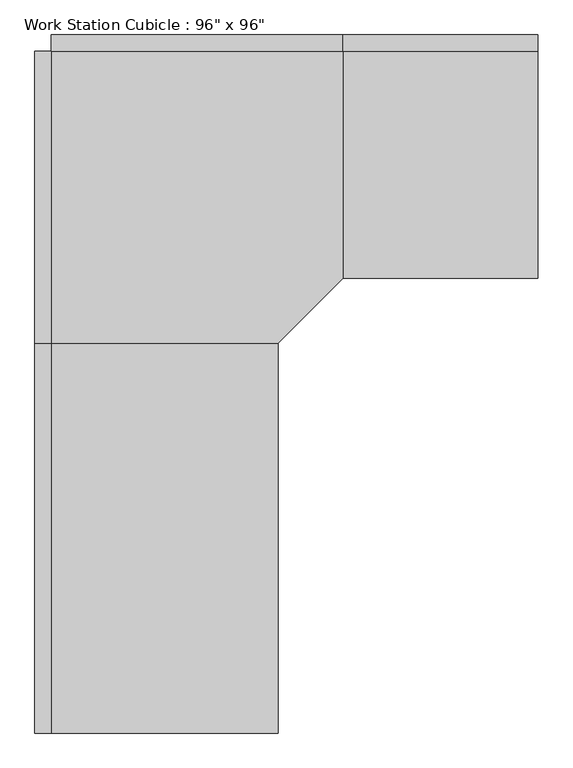
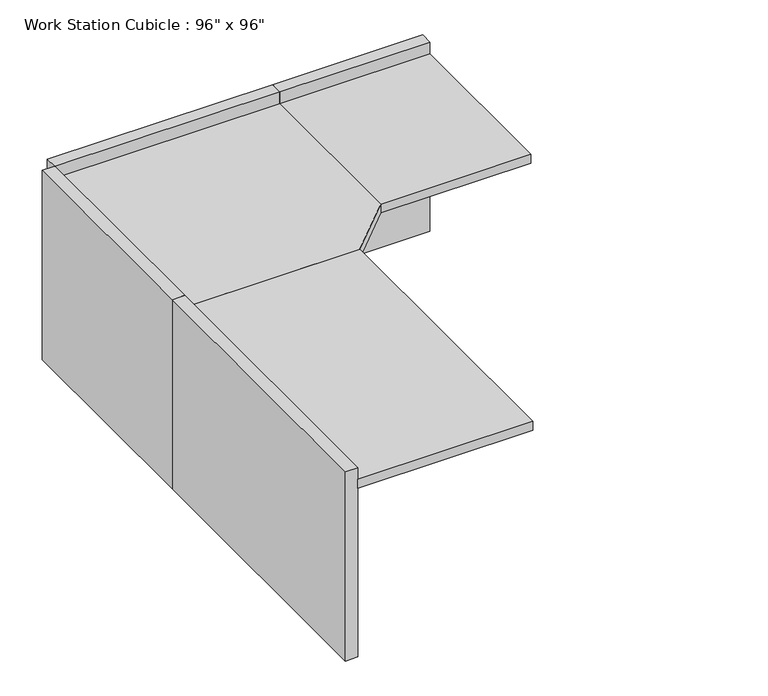
"""IFC4 building model written with IfcOpenShell, lengths in millimetres: furniture geometry."""

from ifc_helpers import new_model, si_unit, frame, origin, origin_with_axes, place, context, project, spatial, polyline, outline, extrude, source, transform, mapped, element, save


def furniture_d6d39c5b(model_context):
    return source(origin(), model_context, "Body", "SweptSolid", [
        extrude(outline(polyline([(-80.9317522, -545.8230076), (833.4682478, -545.8230076), (833.4682478, -1257.0230076), (630.2682478, -1460.2230076), (-80.9317522, -1460.2230076), (-80.9317522, -545.8230076)])), frame((0.0, 0.0, 723.9), z_axis=(0.0, 0.0, 1.0), x_axis=(1.0, 0.0, 0.0)), (0.0, 0.0, 1.0), 38.1),
        extrude(outline(polyline([(630.2682478, -2679.4230076), (-80.9317522, -2679.4230076), (-80.9317522, -1460.2230076), (630.2682478, -1460.2230076), (630.2682478, -2679.4230076)])), frame((0.0, 0.0, 723.9), z_axis=(0.0, 0.0, 1.0), x_axis=(1.0, 0.0, 0.0)), (0.0, 0.0, 1.0), 38.1),
        extrude(outline(polyline([(1443.0682478, -1257.0230076), (833.4682478, -1257.0230076), (833.4682478, -545.8230076), (1443.0682478, -545.8230076), (1443.0682478, -1257.0230076)])), frame((0.0, 0.0, 723.9), z_axis=(0.0, 0.0, 1.0), x_axis=(1.0, 0.0, 0.0)), (0.0, 0.0, 1.0), 38.1),
        extrude(outline(polyline([(1443.0682478, -545.8230076), (833.4682478, -545.8230076), (833.4682478, -495.0230076), (1443.0682478, -495.0230076), (1443.0682478, -545.8230076)])), origin_with_axes(), (0.0, 0.0, 1.0), 812.8),
        extrude(outline(polyline([(833.4682478, -545.8230076), (-80.9317522, -545.8230076), (-80.9317522, -495.0230076), (833.4682478, -495.0230076), (833.4682478, -545.8230076)])), origin_with_axes(), (0.0, 0.0, 1.0), 812.8),
        extrude(outline(polyline([(-80.9317522, -1460.2230076), (-131.7317522, -1460.2230076), (-131.7317522, -545.8230076), (-80.9317522, -545.8230076), (-80.9317522, -1460.2230076)])), origin_with_axes(), (0.0, 0.0, 1.0), 812.8),
        extrude(outline(polyline([(-80.9317522, -2679.4230076), (-131.7317522, -2679.4230076), (-131.7317522, -1460.2230076), (-80.9317522, -1460.2230076), (-80.9317522, -2679.4230076)])), origin_with_axes(), (0.0, 0.0, 1.0), 812.8),
    ])


if __name__ == "__main__":
    model = new_model("IFC4")
    model_context = context("Model", 3, world=origin())
    ifc_project = project(units=[si_unit("LENGTHUNIT", "METRE", prefix="MILLI")], contexts=[model_context])
    site = spatial("IfcSite", under=ifc_project)
    building = spatial("IfcBuilding", under=site)
    placement = place(None, origin())
    furniture_shape = furniture_d6d39c5b(model_context)
    element("IfcFurniture", 1, ObjectType="Work Station Cubicle : 96\" x 96\"", at=placement, inside=building, context=model_context, shape_type="MappedRepresentation", body=[
        mapped(furniture_shape, transform((0.0, 0.0, 0.0), x_axis=(1.0, 0.0, 0.0), y_axis=(0.0, 1.0, 0.0), z_axis=(0.0, 0.0, 1.0))),
    ])
    save(model, "model.ifc")

# Revit data of these elements
# Type "Work Station Cubicle : 96\" x 96\""
#   Assembly Code = "E2020"
#   Desktop Height = 2' - 6"
#   Desktop1 Width = 2' - 4"
#   Desktop2 Width = 2' - 4"
#   Panel Height = 2' - 8"
#   Panel1 Length = 4' - 0"
#   Panel2 Length = 2' - 0"
#   Cube Panel Material = Textile - Light Gray
#   Work Top Material = Laminate, Ivory, Matte
#   Default Elevation = 0
# Element 1 (IfcFurniture, "Work Station Cubicle : 96\" x 96\"")
#   Materials on its faces: "Textile - Light Gray", "Laminate, Ivory, Matte"
# Materials
#   "Textile - Light Gray": class "Fabric", colour RGB 204 204 204, transparency 0
#   "Laminate, Ivory, Matte": class "Plastic", colour RGB 247 247 239, transparency 0, Description = "Plastic Laminate - Ivory, Matte", Cost = 0
